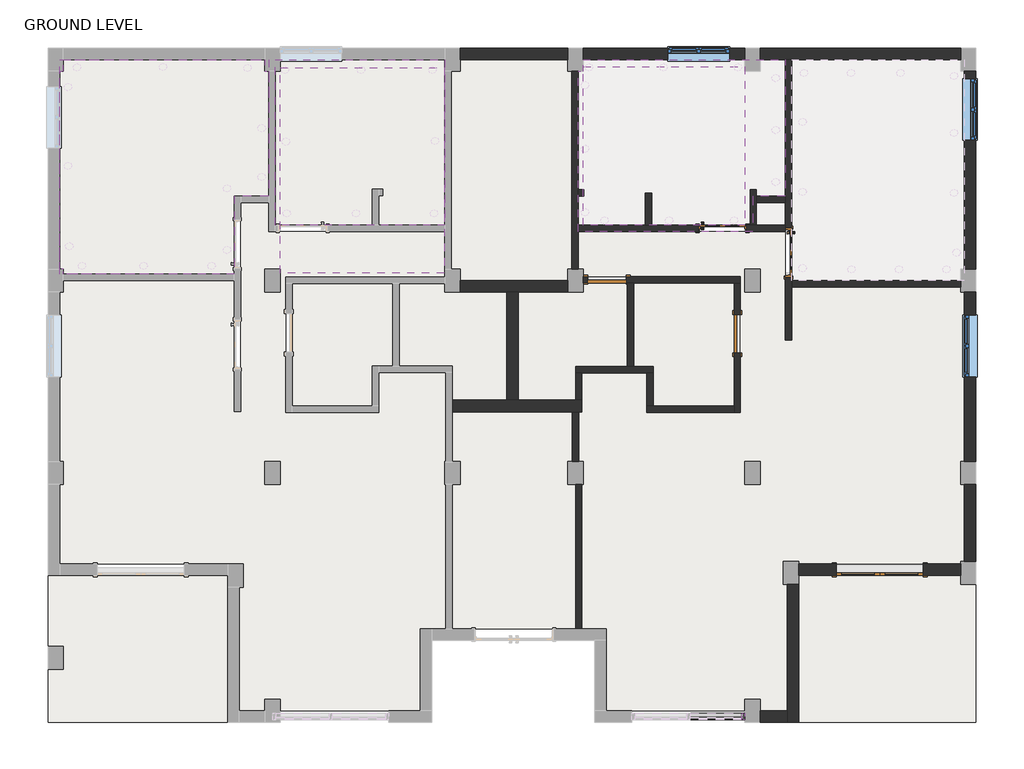
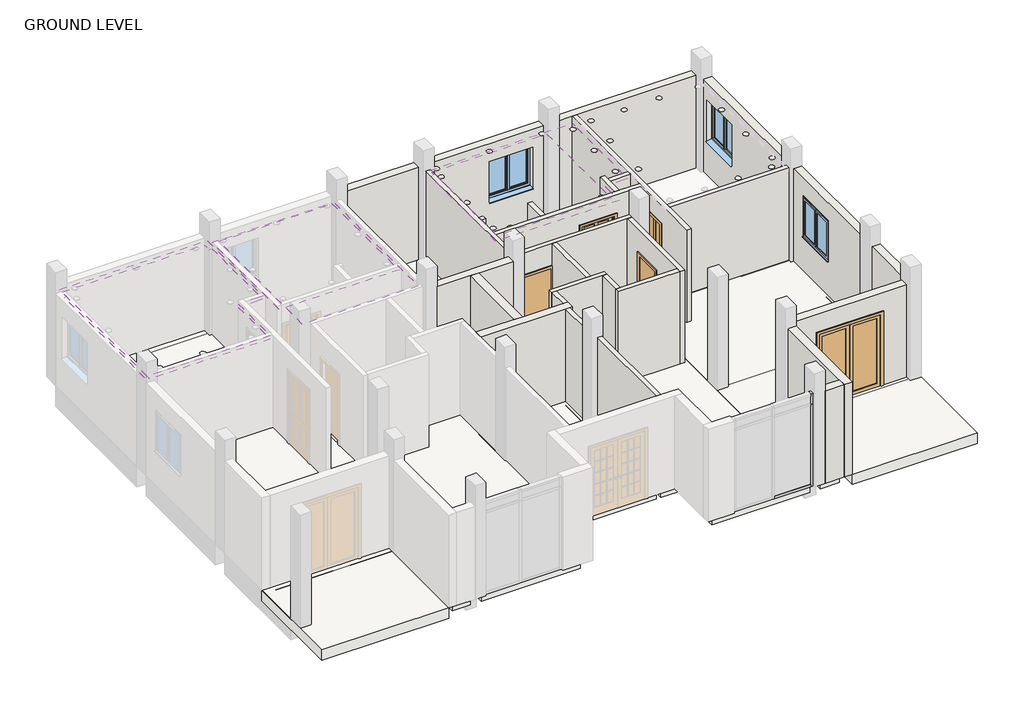
# One storey, part 2 of 5: 29 walls, 7 slabs, 6 coverings, 5 doors, 3 members, 3 windows.
"""IFC4 building model written with IfcOpenShell, lengths in millimetres."""

from ifc_helpers import new_model, si_unit, frame, origin, origin_with_axes, place, context, project, spatial, polyline, outline, extrude, faceted_brep, transform, mapped, element, save
from components import door_e52a3823, door_68a706ac, door_1fe7f57d, member_a1c24a98, member_ee409385, member_3c3dc66a, w2_0001_windows_4_x_4_9dec5fc7

model = new_model("IFC4")

# Units and contexts
model_context = context("Model", 3, world=origin())
ifc_project = project(units=[si_unit("LENGTHUNIT", "METRE", prefix="MILLI")], contexts=[model_context])

# Site, building, storey
site = spatial("IfcSite", under=ifc_project)
building = spatial("IfcBuilding", under=site)
storey = spatial("IfcBuildingStorey", under=building, Name="GROUND LEVEL", Elevation=0.0)

# Coverings
placement = place(None, origin())
element("IfcCovering", 1, ObjectType="white ceiling 6\"", at=placement, inside=storey, context=model_context, shape_type="SweptSolid", body=[
    extrude(outline(polyline([(-8916.1786397, -5702.2620333), (-8916.1786397, -1452.2061634), (-4776.7175798, -1452.2061634), (-4776.7175798, -4153.3104011), (-5462.5175798, -4153.3104011), (-5462.5175798, -5702.2620333), (-8916.1786397, -5702.2620333)])), frame((0.0, 0.0, 2641.6), z_axis=(0.0, 0.0, 1.0), x_axis=(1.0, 0.0, 0.0)), (0.0, 0.0, 1.0), 41.275),
])
element("IfcCovering", 2, ObjectType="white ceiling 6\"", at=placement, inside=storey, context=model_context, shape_type="SweptSolid", body=[
    extrude(outline(polyline([(-4852.9175798, -1452.2061634), (-4852.9175798, -1680.8061634), (-4776.7175798, -1680.8061634), (-4776.7175798, -4153.3104011), (-5462.5175798, -4153.3104011), (-5462.5175798, -5702.2620333), (-8839.9786397, -5702.2620333), (-8839.9786397, -5600.6620333), (-8916.1786397, -5600.6620333), (-8916.1786397, -1680.8061634), (-8839.9786397, -1680.8061634), (-8839.9786397, -1452.2061634), (-4852.9175798, -1452.2061634)]), holes=[polyline([(-8611.3786397, -5397.4620333), (-5767.3175798, -5397.4620333), (-5767.3175798, -3848.5104011), (-5081.5175798, -3848.5104011), (-5081.5175798, -1757.0061634), (-8611.3786397, -1757.0061634), (-8611.3786397, -5397.4620333)])]), frame((0.0, 0.0, 2540.0), z_axis=(0.0, 0.0, 1.0), x_axis=(1.0, 0.0, 0.0)), (0.0, 0.0, 1.0), 41.275),
])
element("IfcCovering", 3, ObjectType="white ceiling 6\"", at=placement, inside=storey, context=model_context, shape_type="SweptSolid", body=[
    extrude(outline(polyline([(-1296.9175798, -1452.2061634), (-1296.9175798, -4728.8061634), (-4649.7175798, -4728.8061634), (-4649.7175798, -1452.2061634), (-1296.9175798, -1452.2061634)]), holes=[polyline([(-1677.9175798, -1833.2061634), (-4268.7175798, -1833.2061634), (-4268.7175798, -4347.8061634), (-1677.9175798, -4347.8061634), (-1677.9175798, -1833.2061634)])]), frame((0.0, 0.0, 2540.0), z_axis=(0.0, 0.0, 1.0), x_axis=(1.0, 0.0, 0.0)), (0.0, 0.0, 1.0), 41.275),
])
element("IfcCovering", 4, ObjectType="white ceiling 6\"", at=placement, inside=storey, context=model_context, shape_type="SweptSolid", body=[
    extrude(outline(polyline([(5446.7824202, -1452.2061634), (5446.7824202, -1680.8061634), (5446.7824202, -4157.3061634), (4798.34348, -4157.3061634), (4798.34348, -4857.7120333), (1344.6824202, -4857.7120333), (1344.6824202, -1680.8061634), (1446.2824202, -1680.8061634), (1446.2824202, -1452.2061634), (5446.7824202, -1452.2061634)]), holes=[polyline([(1674.8824202, -4551.0061634), (4518.94348, -4551.0061634), (4518.94348, -3848.5104011), (5065.7824202, -3848.5104011), (5065.7824202, -1757.0061634), (1674.8824202, -1757.0061634), (1674.8824202, -4551.0061634)])]), frame((0.0, 0.0, 2540.0), z_axis=(0.0, 0.0, 1.0), x_axis=(1.0, 0.0, 0.0)), (0.0, 0.0, 1.0), 41.275),
])
element("IfcCovering", 5, ObjectType="white ceiling 6\"", at=placement, inside=storey, context=model_context, shape_type="SweptSolid", body=[
    extrude(outline(polyline([(1446.2303381, -4730.7120333), (1446.2303381, -1598.2561634), (4646.6303381, -1598.2561634), (4646.6303381, -4730.7120333), (1446.2303381, -4730.7120333)])), frame((0.0, 0.0, 2590.8), z_axis=(0.0, 0.0, 1.0), x_axis=(1.0, 0.0, 0.0)), (0.0, 0.0, 1.0), 41.275),
])
element("IfcCovering", 6, ObjectType="white ceiling 6\"", at=placement, inside=storey, context=model_context, shape_type="SweptSolid", body=[
    extrude(outline(polyline([(-4547.3786397, -5676.8620333), (-4547.3786397, -1617.3061634), (-1303.2675798, -1617.3061634), (-1303.2675798, -5676.8620333), (-4547.3786397, -5676.8620333)])), frame((0.0, 0.0, 2641.6), z_axis=(0.0, 0.0, 1.0), x_axis=(1.0, 0.0, 0.0)), (0.0, 0.0, 1.0), 41.275),
])

# Doors
door_shape = door_e52a3823(model_context)
element("IfcDoor", 7, ObjectType="Door-Double-Glass : 68\" x 84\"", at=placement, inside=storey, context=model_context, shape_type="MappedRepresentation", body=[
    mapped(door_shape, transform((7313.6824202, -11554.5807833, 0.0), x_axis=(-1.0, 0.0, 0.0), y_axis=(0.0, -1.0, 0.0), z_axis=(0.0, 0.0, 1.0))),
])
door_2_shape = door_68a706ac(model_context)
element("IfcDoor", 8, ObjectType="Door-Interior-Single-4_Panel-Wood : 36\" x 84\"", at=placement, inside=storey, context=model_context, shape_type="MappedRepresentation", body=[
    mapped(door_2_shape, transform((4202.1824202, -4789.1311634, 0.0), x_axis=(1.0, 0.0, 0.0), y_axis=(0.0, 1.0, 0.0), z_axis=(0.0, 0.0, 1.0))),
])
element("IfcDoor", 9, ObjectType="Door-Interior-Single-4_Panel-Wood : 36\" x 84\"", at=placement, inside=storey, context=model_context, shape_type="MappedRepresentation", body=[
    mapped(door_2_shape, transform((5513.4574202, -5274.9061634, 0.0), x_axis=(0.0, -1.0, 0.0), y_axis=(1.0, 0.0, 0.0), z_axis=(0.0, 0.0, 1.0))),
])
door_3_shape = door_1fe7f57d(model_context)
element("IfcDoor", 10, ObjectType="Single-Flush : 30\" x 80\"", at=placement, inside=storey, context=model_context, shape_type="MappedRepresentation", body=[
    mapped(door_3_shape, transform((1916.1824202, -5810.8691591, 0.0), x_axis=(-1.0, 0.0, 0.0), y_axis=(0.0, -1.0, 0.0), z_axis=(0.0, 0.0, 1.0))),
])
element("IfcDoor", 11, ObjectType="Single-Flush : 30\" x 80\"", at=placement, inside=storey, context=model_context, shape_type="MappedRepresentation", body=[
    mapped(door_3_shape, transform((4494.2824202, -6877.6691591, 0.0), x_axis=(0.0, 1.0, 0.0), y_axis=(-1.0, 0.0, 0.0), z_axis=(0.0, 0.0, 1.0))),
])

# Members
member_shape = member_a1c24a98(model_context)
element("IfcMember", 12, ObjectType="Rectangular Mullion : 2.5\" x 5\" rectangular", at=placement, inside=storey, context=model_context, shape_type="MappedRepresentation", body=[
    mapped(member_shape, transform((4583.1824202, -14462.5402089, 0.0), x_axis=(0.0, 0.0, -1.0), y_axis=(0.0, 1.0, 0.0), z_axis=(1.0, 0.0, 0.0))),
])
member_2_shape = member_ee409385(model_context)
element("IfcMember", 13, ObjectType="Rectangular Mullion : 2.5\" x 5\" rectangular", at=placement, inside=storey, context=model_context, shape_type="MappedRepresentation", body=[
    mapped(member_2_shape, transform((4646.6824202, -14462.5402089, 2438.4), x_axis=(1.0, 0.0, 0.0), y_axis=(0.0, 1.0, 0.0), z_axis=(0.0, 0.0, 1.0))),
])
member_3_shape = member_3c3dc66a(model_context)
element("IfcMember", 14, ObjectType="Rectangular Mullion : 2.5\" x 5\" rectangular", at=placement, inside=storey, context=model_context, shape_type="MappedRepresentation", body=[
    mapped(member_3_shape, transform((4646.6824202, -14462.5402089, 2743.2), x_axis=(1.0, 0.0, 0.0), y_axis=(0.0, 1.0, 0.0), z_axis=(0.0, 0.0, 1.0))),
])

# Slabs
element("IfcSlab", 15, ObjectType="TILE FLOORING 1'", at=placement, inside=storey, context=model_context, shape_type="SweptSolid", body=[
    extrude(outline(polyline([(-4315.5950401, -8312.1120333), (-4315.5950401, -5885.8942903), (-2325.6175798, -5885.8942903), (-2325.6175798, -7524.7120333), (-2728.0950401, -7524.7120333), (-2728.0950401, -8312.1120333), (-4315.5950401, -8312.1120333)])), frame((0.0, 0.0, -304.8), z_axis=(0.0, 0.0, 1.0), x_axis=(1.0, 0.0, 0.0)), (0.0, 0.0, 1.0), 304.8),
    extrude(outline(polyline([(-1296.9175798, -5885.8942903), (-1296.9175798, -6057.8620333), (-65.0175798, -6057.8620333), (-65.0175798, -8197.8120333), (-1144.5175798, -8197.8120333), (-1144.5175798, -7524.7120333), (-2198.6175798, -7524.7120333), (-2198.6175798, -5885.8942903), (-1296.9175798, -5885.8942903)])), frame((0.0, 0.0, -304.8), z_axis=(0.0, 0.0, 1.0), x_axis=(1.0, 0.0, 0.0)), (0.0, 0.0, 1.0), 304.8),
    extrude(outline(polyline([(1293.8824202, -8197.8120333), (163.5824202, -8197.8120333), (163.5824202, -6057.8620333), (1446.2824202, -6057.8620333), (1446.2824202, -5874.3691591), (2322.5824202, -5874.3691591), (2322.5824202, -7533.8890971), (1293.8824202, -7533.8890971), (1293.8824202, -8197.8120333)])), frame((0.0, 0.0, -304.8), z_axis=(0.0, 0.0, 1.0), x_axis=(1.0, 0.0, 0.0)), (0.0, 0.0, 1.0), 304.8),
    extrude(outline(polyline([(2449.5824202, -7533.8890971), (2449.5824202, -5874.3691591), (4430.7824202, -5874.3691591), (4430.7824202, -8312.7691591), (2830.5824202, -8312.7691591), (2830.5824202, -7533.8890971), (2449.5824202, -7533.8890971)])), frame((0.0, 0.0, -304.8), z_axis=(0.0, 0.0, 1.0), x_axis=(1.0, 0.0, 0.0)), (0.0, 0.0, 1.0), 304.8),
])
element("IfcSlab", 16, ObjectType="flooring 1'", at=placement, inside=storey, context=model_context, shape_type="SweptSolid", body=[
    extrude(outline(polyline([(-8916.1786397, -11442.6620333), (-8916.1786397, -9867.8620333), (-8839.9786397, -9867.8620333), (-8839.9786397, -9410.6620333), (-8916.1786397, -9410.6620333), (-8916.1786397, -6057.8620333), (-8839.9786397, -6057.8620333), (-8839.9786397, -5829.2620333), (-5462.5175798, -5829.2620333), (-5462.5175798, -8420.0620333), (-5335.5175798, -8420.0620333), (-5335.5175798, -4280.3104011), (-4776.7175798, -4280.3104011), (-4776.7175798, -4855.8061634), (-1296.9175798, -4855.8061634), (-1296.9175798, -5600.6620333), (-1296.9175798, -5758.8942903), (-4442.5950401, -5758.8942903), (-4442.5950401, -8439.1120333), (-2601.0950401, -8439.1120333), (-2601.0950401, -7651.7120333), (-1271.5175798, -7651.7120333), (-1271.5175798, -9410.6620333), (-1296.9175798, -9410.6620333), (-1296.9175798, -9867.8620333), (-1271.5175798, -9867.8620333), (-1271.5175798, -12722.6402089), (-1779.5175798, -12722.6402089), (-1779.5175798, -14348.2402089), (-4548.1175798, -14348.2402089), (-4548.1175798, -14119.6402089), (-4852.9175798, -14119.6402089), (-4852.9175798, -14348.2402089), (-5360.9175798, -14348.2402089), (-5360.9175798, -11899.8620333), (-5284.7175798, -11899.8620333), (-5284.7175798, -11442.6620333), (-5589.5175798, -11442.6620333), (-8916.1786397, -11442.6620333)])), frame((0.0, 0.0, -304.8), z_axis=(0.0, 0.0, 1.0), x_axis=(1.0, 0.0, 0.0)), (0.0, 0.0, 1.0), 304.8),
])
element("IfcSlab", 17, ObjectType="flooring 1'", at=placement, inside=storey, context=model_context, shape_type="SweptSolid", body=[
    extrude(outline(polyline([(5446.7824202, -4855.8061634), (5446.7824202, -6583.0061634), (5573.7824202, -6583.0061634), (5573.7824202, -5956.2620333), (8913.8824202, -5956.2620333), (8913.8824202, -6057.8620333), (8990.0824202, -6057.8620333), (8990.0824202, -9410.6620333), (8913.8824202, -9410.6620333), (8913.8824202, -9867.8620333), (8990.0824202, -9867.8620333), (8990.0824202, -11391.8620333), (8913.8824202, -11391.8620333), (8913.8824202, -11442.6620333), (5713.4824202, -11442.6620333), (5713.4824202, -11391.8620333), (5408.6824202, -11391.8620333), (5408.6824202, -11849.0620333), (5484.8824202, -11849.0620333), (5484.8824202, -14348.2402089), (4951.4824202, -14348.2402089), (4951.4824202, -14119.6402089), (4646.6824202, -14119.6402089), (4646.6824202, -14348.2402089), (1903.4824202, -14348.2402089), (1903.4824202, -12722.6402089), (1420.8824202, -12722.6402089), (1420.8824202, -9867.8620333), (1446.2824202, -9867.8620333), (1446.2824202, -9410.6620333), (1357.3824202, -9410.6620333), (1357.3824202, -8426.4120333), (1420.8824202, -8426.4120333), (1420.8824202, -7660.8890971), (2703.5824202, -7660.8890971), (2703.5824202, -8439.7691591), (4557.7824202, -8439.7691591), (4557.7824202, -5747.3691591), (1446.2824202, -5747.3691591), (1446.2824202, -5600.6620333), (1344.6824202, -5600.6620333), (1344.6824202, -4855.8061634), (5446.7824202, -4855.8061634)])), frame((0.0, 0.0, -304.8), z_axis=(0.0, 0.0, 1.0), x_axis=(1.0, 0.0, 0.0)), (0.0, 0.0, 1.0), 304.8),
])
element("IfcSlab", 18, ObjectType="flooring 1'", at=placement, inside=storey, context=model_context, shape_type="SweptSolid", body=[
    extrude(outline(polyline([(-8839.9786397, -1680.8061634), (-8839.9786397, -1452.2061634), (-4852.9175798, -1452.2061634), (-4852.9175798, -1680.8061634), (-4776.7175798, -1680.8061634), (-4776.7175798, -4153.3104011), (-5462.5175798, -4153.3104011), (-5462.5175798, -5702.2620333), (-8839.9786397, -5702.2620333), (-8839.9786397, -5600.6620333), (-8916.1786397, -5600.6620333), (-8916.1786397, -1680.8061634), (-8839.9786397, -1680.8061634)])), frame((0.0, 0.0, -304.8), z_axis=(0.0, 0.0, 1.0), x_axis=(1.0, 0.0, 0.0)), (0.0, 0.0, 1.0), 304.8),
    extrude(outline(polyline([(-2732.0175798, -4728.8061634), (-4649.7175798, -4728.8061634), (-4649.7175798, -1680.8061634), (-4548.1175798, -1680.8061634), (-4548.1175798, -1452.2061634), (-1296.9175798, -1452.2061634), (-1296.9175798, -4728.8061634), (-2605.0175798, -4728.8061634), (-2605.0175798, -4144.6061634), (-2516.1175798, -4144.6061634), (-2516.1175798, -4017.6061634), (-2732.0175798, -4017.6061634), (-2732.0175798, -4728.8061634)])), frame((0.0, 0.0, -304.8), z_axis=(0.0, 0.0, 1.0), x_axis=(1.0, 0.0, 0.0)), (0.0, 0.0, 1.0), 304.8),
])
element("IfcSlab", 19, ObjectType="flooring 1'", at=placement, inside=storey, context=model_context, shape_type="SweptSolid", body=[
    extrude(outline(polyline([(1141.4824202, -1452.2061634), (1141.4824202, -1680.8061634), (1217.6824202, -1680.8061634), (1217.6824202, -5600.6620333), (1141.4824202, -5600.6620333), (1141.4824202, -5829.2620333), (-992.1175798, -5829.2620333), (-992.1175798, -5600.6620333), (-1169.9175798, -5600.6620333), (-1169.9175798, -1680.8061634), (-992.1175798, -1680.8061634), (-992.1175798, -1452.2061634), (1141.4824202, -1452.2061634)])), frame((0.0, 0.0, -304.8), z_axis=(0.0, 0.0, 1.0), x_axis=(1.0, 0.0, 0.0)), (0.0, 0.0, 1.0), 304.8),
])
element("IfcSlab", 20, ObjectType="flooring 1'", at=placement, inside=storey, context=model_context, shape_type="SweptSolid", body=[
    extrude(outline(polyline([(1293.8824202, -12722.6402089), (-1144.5175798, -12722.6402089), (-1144.5175798, -9867.8620333), (-992.1175798, -9867.8620333), (-992.1175798, -9410.6620333), (-1144.5175798, -9410.6620333), (-1144.5175798, -8426.4120333), (1230.3824202, -8426.4120333), (1230.3824202, -9410.6620333), (1141.4824202, -9410.6620333), (1141.4824202, -9867.8620333), (1293.8824202, -9867.8620333), (1293.8824202, -12722.6402089)])), frame((0.0, 0.0, -304.8), z_axis=(0.0, 0.0, 1.0), x_axis=(1.0, 0.0, 0.0)), (0.0, 0.0, 1.0), 304.8),
])
element("IfcSlab", 21, ObjectType="flooring 1'", at=placement, inside=storey, context=model_context, shape_type="SweptSolid", body=[
    extrude(outline(polyline([(-5589.5175798, -11671.2620333), (-5589.5175798, -14576.8402089), (-9144.7786397, -14576.8402089), (-9144.7786397, -11671.2620333), (-5589.5175798, -11671.2620333)])), frame((0.0, 0.0, -304.8), z_axis=(0.0, 0.0, 1.0), x_axis=(1.0, 0.0, 0.0)), (0.0, 0.0, 1.0), 304.8),
    extrude(outline(polyline([(9218.6824202, -11671.2620333), (9218.6824202, -14576.8402089), (5713.4824202, -14576.8402089), (5713.4824202, -11671.2620333), (9218.6824202, -11671.2620333)])), frame((0.0, 0.0, -304.8), z_axis=(0.0, 0.0, 1.0), x_axis=(1.0, 0.0, 0.0)), (0.0, 0.0, 1.0), 304.8),
])

# Walls
element("IfcWall", 22, ObjectType="EXTERIOR WALL 9\"", at=placement, inside=storey, context=model_context, shape_type="SweptSolid", body=[
    extrude(outline(polyline([(1141.4824202, -1452.2061634), (-992.1175798, -1452.2061634), (-992.1175798, -1223.6061634), (1141.4824202, -1223.6061634), (1141.4824202, -1452.2061634)])), origin_with_axes(), (0.0, 0.0, 1.0), 2743.2),
])
element("IfcWall", 23, ObjectType="EXTERIOR WALL 9\"", at=placement, inside=storey, context=model_context, shape_type="SweptSolid", body=[
    extrude(outline(polyline([(0.0, 1446.2824202), (0.0, 4646.6824202), (2743.2, 4646.6824202), (2743.2, 1446.2824202), (0.0, 1446.2824202)]), holes=[polyline([(1000.0, 4341.8824202), (1000.0, 3122.6824202), (2219.2, 3122.6824202), (2219.2, 4341.8824202), (1000.0, 4341.8824202)])]), frame((0.0, -1452.2061634, 0.0), z_axis=(0.0, 1.0, 0.0), x_axis=(0.0, 0.0, 1.0)), (0.0, 0.0, 1.0), 228.6),
])
element("IfcWall", 24, ObjectType="EXTERIOR WALL 9\"", at=placement, inside=storey, context=model_context, shape_type="Brep", body=[
    faceted_brep([(4951.4824202, -1452.2061634, 0.0), (5446.7824202, -1452.2061634, 0.0), (5573.7824202, -1452.2061634, 0.0), (8913.8824202, -1452.2061634, 0.0), (8913.8824202, -1452.2061634, 2743.2), (5573.7824202, -1452.2061634, 2743.2), (5446.7824202, -1452.2061634, 2743.2), (4951.4824202, -1452.2061634, 2743.2), (4951.4824202, -1223.6061634, 0.0), (4951.4824202, -1223.6061634, 2743.2), (8913.8824202, -1223.6061634, 2743.2), (8913.8824202, -1223.6061634, 0.0)], [[[0, 1, 2, 3, 4, 5, 6, 7]], [[8, 9, 10, 11]], [[3, 2, 1, 0, 8, 11]], [[4, 3, 11, 10]], [[7, 6, 5, 4, 10, 9]], [[0, 7, 9, 8]]]),
])
element("IfcWall", 25, ObjectType="EXTERIOR WALL 9\"", at=placement, inside=storey, context=model_context, shape_type="SweptSolid", body=[
    extrude(outline(polyline([(-1680.8061634, 0.0), (-5600.6620333, 0.0), (-5600.6620333, 2743.2), (-1680.8061634, 2743.2), (-1680.8061634, 0.0)]), holes=[polyline([(-3052.4061634, 1000.0), (-1833.2061634, 1000.0), (-1833.2061634, 2219.2), (-3052.4061634, 2219.2), (-3052.4061634, 1000.0)])]), frame((8990.0824202, 0.0, 0.0), z_axis=(1.0, 0.0, 0.0), x_axis=(0.0, 1.0, 0.0)), (0.0, 0.0, 1.0), 228.6),
])
element("IfcWall", 26, ObjectType="EXTERIOR WALL 9\"", at=placement, inside=storey, context=model_context, shape_type="SweptSolid", body=[
    extrude(outline(polyline([(-6057.8620333, 0.0), (-9410.6620333, 0.0), (-9410.6620333, 2743.2), (-6057.8620333, 2743.2), (-6057.8620333, 0.0)]), holes=[polyline([(-6515.0620333, 1000.0), (-6515.0620333, 2219.2), (-7734.2620333, 2219.2), (-7734.2620333, 1000.0), (-6515.0620333, 1000.0)])]), frame((8990.0824202, 0.0, 0.0), z_axis=(1.0, 0.0, 0.0), x_axis=(0.0, 1.0, 0.0)), (0.0, 0.0, 1.0), 228.6),
])
element("IfcWall", 27, ObjectType="EXTERIOR WALL 9\"", at=placement, inside=storey, context=model_context, shape_type="SweptSolid", body=[
    extrude(outline(polyline([(8990.0824202, -11391.8620333), (8990.0824202, -9867.8620333), (9218.6824202, -9867.8620333), (9218.6824202, -11391.8620333), (8990.0824202, -11391.8620333)])), origin_with_axes(), (0.0, 0.0, 1.0), 2743.2),
])
element("IfcWall", 28, ObjectType="EXTERIOR WALL 9\"", at=placement, inside=storey, context=model_context, shape_type="SweptSolid", body=[
    extrude(outline(polyline([(2743.2, 5713.4824202), (0.0, 5713.4824202), (0.0, 6450.0824202), (2133.6, 6450.0824202), (2133.6, 8177.2824202), (0.0, 8177.2824202), (0.0, 8913.8824202), (2743.2, 8913.8824202), (2743.2, 5713.4824202)])), frame((0.0, -11671.2620333, 0.0), z_axis=(0.0, 1.0, 0.0), x_axis=(0.0, 0.0, 1.0)), (0.0, 0.0, 1.0), 228.6),
])
element("IfcWall", 29, ObjectType="EXTERIOR WALL 9\"", at=placement, inside=storey, context=model_context, shape_type="Brep", body=[
    faceted_brep([(5484.8824202, -11849.0620333, 0.0), (5484.8824202, -14348.2402089, 0.0), (5484.8824202, -14576.8402089, 0.0), (5484.8824202, -14576.8402089, 2743.2), (5484.8824202, -14348.2402089, 2743.2), (5484.8824202, -11849.0620333, 2743.2), (5713.4824202, -11849.0620333, 0.0), (5713.4824202, -11849.0620333, 2743.2), (5713.4824202, -14576.8402089, 2743.2), (5713.4824202, -14576.8402089, 0.0)], [[[0, 1, 2, 3, 4, 5]], [[6, 7, 8, 9]], [[2, 1, 0, 6, 9]], [[5, 4, 3, 8, 7]], [[0, 5, 7, 6]], [[3, 2, 9, 8]]]),
])
element("IfcWall", 30, ObjectType="EXTERIOR WALL 9\"", at=placement, inside=storey, context=model_context, shape_type="SweptSolid", body=[
    extrude(outline(polyline([(5484.8824202, -14576.8402089), (4951.4824202, -14576.8402089), (4951.4824202, -14348.2402089), (5484.8824202, -14348.2402089), (5484.8824202, -14576.8402089)])), origin_with_axes(), (0.0, 0.0, 1.0), 2743.2),
])
element("IfcWall", 31, ObjectType="EXTERIOR WALL 9\"", at=placement, inside=storey, context=model_context, shape_type="Brep", body=[
    faceted_brep([(1141.4824202, -5829.2620333, 0.0), (-992.1175798, -5829.2620333, 0.0), (-992.1175798, -5829.2620333, 2743.2), (1141.4824202, -5829.2620333, 2743.2), (1141.4824202, -6057.8620333, 0.0), (1141.4824202, -6057.8620333, 2743.2), (163.5824202, -6057.8620333, 2743.2), (-65.0175798, -6057.8620333, 2743.2), (-992.1175798, -6057.8620333, 2743.2), (-992.1175798, -6057.8620333, 0.0), (-65.0175798, -6057.8620333, 0.0), (163.5824202, -6057.8620333, 0.0)], [[[0, 1, 2, 3]], [[4, 5, 6, 7, 8, 9, 10, 11]], [[1, 0, 4, 11, 10, 9]], [[2, 1, 9, 8]], [[3, 2, 8, 7, 6, 5]], [[0, 3, 5, 4]]]),
])
element("IfcWall", 32, ObjectType="EXTERIOR WALL 9\"", at=placement, inside=storey, context=model_context, shape_type="SweptSolid", body=[
    extrude(outline(polyline([(-65.0175798, -8197.8120333), (-65.0175798, -6057.8620333), (163.5824202, -6057.8620333), (163.5824202, -8197.8120333), (-65.0175798, -8197.8120333)])), origin_with_axes(), (0.0, 0.0, 1.0), 2743.2),
])
element("IfcWall", 33, ObjectType="EXTERIOR WALL 9\"", at=placement, inside=storey, context=model_context, shape_type="Brep", body=[
    faceted_brep([(-1144.5175798, -8426.4120333, 0.0), (1230.3824202, -8426.4120333, 0.0), (1357.3824202, -8426.4120333, 0.0), (1420.8824202, -8426.4120333, 0.0), (1420.8824202, -8426.4120333, 2743.2), (1357.3824202, -8426.4120333, 2743.2), (1230.3824202, -8426.4120333, 2743.2), (-1144.5175798, -8426.4120333, 2743.2), (-1144.5175798, -8197.8120333, 0.0), (-1144.5175798, -8197.8120333, 2743.2), (-65.0175798, -8197.8120333, 2743.2), (163.5824202, -8197.8120333, 2743.2), (1293.8824202, -8197.8120333, 2743.2), (1420.8824202, -8197.8120333, 2743.2), (1420.8824202, -8197.8120333, 0.0), (1293.8824202, -8197.8120333, 0.0), (163.5824202, -8197.8120333, 0.0), (-65.0175798, -8197.8120333, 0.0)], [[[0, 1, 2, 3, 4, 5, 6, 7]], [[8, 9, 10, 11, 12, 13, 14, 15, 16, 17]], [[3, 2, 1, 0, 8, 17, 16, 15, 14]], [[7, 6, 5, 4, 13, 12, 11, 10, 9]], [[0, 7, 9, 8]], [[4, 3, 14, 13]]]),
])
element("IfcWall", 34, ObjectType="INTERIOR WALL 5\"", at=placement, inside=storey, context=model_context, shape_type="Brep", body=[
    faceted_brep([(1217.6824202, -1680.8061634, 0.0), (1217.6824202, -5600.6620333, 0.0), (1217.6824202, -5600.6620333, 2743.2), (1217.6824202, -1680.8061634, 2743.2), (1344.6824202, -1680.8061634, 0.0), (1344.6824202, -1680.8061634, 2743.2), (1344.6824202, -4030.3061634, 2743.2), (1344.6824202, -4157.3061634, 2743.2), (1344.6824202, -4728.8061634, 2743.2), (1344.6824202, -4855.8061634, 2743.2), (1344.6824202, -5600.6620333, 2743.2), (1344.6824202, -5600.6620333, 0.0), (1344.6824202, -4855.8061634, 0.0), (1344.6824202, -4728.8061634, 0.0), (1344.6824202, -4157.3061634, 0.0), (1344.6824202, -4030.3061634, 0.0)], [[[0, 1, 2, 3]], [[4, 5, 6, 7, 8, 9, 10, 11, 12, 13, 14, 15]], [[1, 0, 4, 15, 14, 13, 12, 11]], [[2, 1, 11, 10]], [[3, 2, 10, 9, 8, 7, 6, 5]], [[0, 3, 5, 4]]]),
])
element("IfcWall", 35, ObjectType="INTERIOR WALL 5\"", at=placement, inside=storey, context=model_context, shape_type="Brep", body=[
    faceted_brep([(5446.7824202, -4855.8061634, 2743.2), (1344.6824202, -4855.8061634, 2743.2), (1344.6824202, -4855.8061634, 0.0), (3719.5824202, -4855.8061634, 0.0), (3719.5824202, -4855.8061634, 2159.0), (4684.7824202, -4855.8061634, 2159.0), (4684.7824202, -4855.8061634, 0.0), (5446.7824202, -4855.8061634, 0.0), (1344.6824202, -4728.8061634, 2743.2), (2678.1824202, -4728.8061634, 2743.2), (2805.1824202, -4728.8061634, 2743.2), (4748.2824202, -4728.8061634, 2743.2), (4875.2824202, -4728.8061634, 2743.2), (5446.7824202, -4728.8061634, 2743.2), (5446.7824202, -4728.8061634, 0.0), (4875.2824202, -4728.8061634, 0.0), (4748.2824202, -4728.8061634, 0.0), (4684.7824202, -4728.8061634, 0.0), (4684.7824202, -4728.8061634, 2159.0), (3719.5824202, -4728.8061634, 2159.0), (3719.5824202, -4728.8061634, 0.0), (2805.1824202, -4728.8061634, 0.0), (2678.1824202, -4728.8061634, 0.0), (1344.6824202, -4728.8061634, 0.0)], [[[0, 1, 2, 3, 4, 5, 6, 7]], [[8, 9, 10, 11, 12, 13, 14, 15, 16, 17, 18, 19, 20, 21, 22, 23]], [[2, 23, 22, 21, 20, 3]], [[14, 7, 6, 17, 16, 15]], [[1, 0, 13, 12, 11, 10, 9, 8]], [[2, 1, 8, 23]], [[0, 7, 14, 13]], [[5, 18, 17, 6]], [[18, 5, 4, 19]], [[19, 4, 3, 20]]]),
])
element("IfcWall", 36, ObjectType="INTERIOR WALL 5\"", at=placement, inside=storey, context=model_context, shape_type="Brep", body=[
    faceted_brep([(4875.2824202, -4728.8061634, 0.0), (4875.2824202, -4284.3061634, 0.0), (4875.2824202, -4157.3061634, 0.0), (4875.2824202, -4030.3061634, 0.0), (4875.2824202, -4030.3061634, 2743.2), (4875.2824202, -4157.3061634, 2743.2), (4875.2824202, -4284.3061634, 2743.2), (4875.2824202, -4728.8061634, 2743.2), (4748.2824202, -4728.8061634, 0.0), (4748.2824202, -4728.8061634, 2743.2), (4748.2824202, -4030.3061634, 2743.2), (4748.2824202, -4030.3061634, 0.0)], [[[0, 1, 2, 3, 4, 5, 6, 7]], [[8, 9, 10, 11]], [[3, 2, 1, 0, 8, 11]], [[4, 3, 11, 10]], [[7, 6, 5, 4, 10, 9]], [[0, 7, 9, 8]]]),
])
element("IfcWall", 37, ObjectType="INTERIOR WALL 5\"", at=placement, inside=storey, context=model_context, shape_type="SweptSolid", body=[
    extrude(outline(polyline([(5446.7824202, -4284.3061634), (4875.2824202, -4284.3061634), (4875.2824202, -4157.3061634), (5446.7824202, -4157.3061634), (5446.7824202, -4284.3061634)])), origin_with_axes(), (0.0, 0.0, 1.0), 2743.2),
])
element("IfcWall", 38, ObjectType="INTERIOR WALL 5\"", at=placement, inside=storey, context=model_context, shape_type="Brep", body=[
    faceted_brep([(5446.7824202, -7002.1061634, 0.0), (5446.7824202, -7002.1061634, 2743.2), (5446.7824202, -4855.8061634, 2743.2), (5446.7824202, -4728.8061634, 2743.2), (5446.7824202, -4284.3061634, 2743.2), (5446.7824202, -4157.3061634, 2743.2), (5446.7824202, -1452.2061634, 2743.2), (5446.7824202, -1452.2061634, 0.0), (5446.7824202, -4157.3061634, 0.0), (5446.7824202, -4284.3061634, 0.0), (5446.7824202, -4728.8061634, 0.0), (5446.7824202, -4792.3061634, 0.0), (5446.7824202, -4792.3061634, 2159.0), (5446.7824202, -5757.5061634, 2159.0), (5446.7824202, -5757.5061634, 0.0), (5573.7824202, -7002.1061634, 2743.2), (5573.7824202, -7002.1061634, 0.0), (5573.7824202, -5956.2620333, 0.0), (5573.7824202, -5829.2620333, 0.0), (5573.7824202, -5757.5061634, 0.0), (5573.7824202, -5757.5061634, 2159.0), (5573.7824202, -4792.3061634, 2159.0), (5573.7824202, -4792.3061634, 0.0), (5573.7824202, -1452.2061634, 0.0), (5573.7824202, -1452.2061634, 2743.2), (5573.7824202, -5829.2620333, 2743.2), (5573.7824202, -5956.2620333, 2743.2)], [[[0, 1, 2, 3, 4, 5, 6, 7, 8, 9, 10, 11, 12, 13, 14]], [[15, 16, 17, 18, 19, 20, 21, 22, 23, 24, 25, 26]], [[16, 0, 14, 19, 18, 17]], [[7, 23, 22, 11, 10, 9, 8]], [[1, 0, 16, 15]], [[6, 5, 4, 3, 2, 1, 15, 26, 25, 24]], [[7, 6, 24, 23]], [[13, 20, 19, 14]], [[20, 13, 12, 21]], [[21, 12, 11, 22]]]),
])
element("IfcWall", 39, ObjectType="INTERIOR WALL 5\"", at=placement, inside=storey, context=model_context, shape_type="SweptSolid", body=[
    extrude(outline(polyline([(5573.7824202, -5829.2620333), (8913.8824202, -5829.2620333), (8913.8824202, -5956.2620333), (5573.7824202, -5956.2620333), (5573.7824202, -5829.2620333)])), origin_with_axes(), (0.0, 0.0, 1.0), 2743.2),
])
element("IfcWall", 40, ObjectType="INTERIOR WALL 5\"", at=placement, inside=storey, context=model_context, shape_type="SweptSolid", body=[
    extrude(outline(polyline([(2805.1824202, -4093.8061634), (2805.1824202, -4728.8061634), (2678.1824202, -4728.8061634), (2678.1824202, -4093.8061634), (2805.1824202, -4093.8061634)])), origin_with_axes(), (0.0, 0.0, 1.0), 2743.2),
])
element("IfcWall", 41, ObjectType="INTERIOR WALL 5\"", at=placement, inside=storey, context=model_context, shape_type="SweptSolid", body=[
    extrude(outline(polyline([(1458.9824202, -4157.3061634), (1344.6824202, -4157.3061634), (1344.6824202, -4030.3061634), (1458.9824202, -4030.3061634), (1458.9824202, -4157.3061634)])), origin_with_axes(), (0.0, 0.0, 1.0), 2743.2),
])
element("IfcWall", 42, ObjectType="INTERIOR WALL 5\"", at=placement, inside=storey, context=model_context, shape_type="Brep", body=[
    faceted_brep([(1535.1824202, -5747.3691591, 2032.0), (1535.1824202, -5747.3691591, 0.0), (1446.2824202, -5747.3691591, 0.0), (1446.2824202, -5747.3691591, 2743.2), (4557.7824202, -5747.3691591, 2743.2), (4557.7824202, -5747.3691591, 0.0), (2297.1824202, -5747.3691591, 0.0), (2297.1824202, -5747.3691591, 2032.0), (1446.2824202, -5874.3691591, 0.0), (1535.1824202, -5874.3691591, 0.0), (1535.1824202, -5874.3691591, 2032.0), (2297.1824202, -5874.3691591, 2032.0), (2297.1824202, -5874.3691591, 0.0), (2322.5824202, -5874.3691591, 0.0), (2449.5824202, -5874.3691591, 0.0), (4430.7824202, -5874.3691591, 0.0), (4557.7824202, -5874.3691591, 0.0), (4557.7824202, -5874.3691591, 2743.2), (4430.7824202, -5874.3691591, 2743.2), (2449.5824202, -5874.3691591, 2743.2), (2322.5824202, -5874.3691591, 2743.2), (1446.2824202, -5874.3691591, 2743.2)], [[[0, 1, 2, 3, 4, 5, 6, 7]], [[8, 9, 10, 11, 12, 13, 14, 15, 16, 17, 18, 19, 20, 21]], [[6, 5, 16, 15, 14, 13, 12]], [[2, 1, 9, 8]], [[3, 2, 8, 21]], [[4, 3, 21, 20, 19, 18, 17]], [[5, 4, 17, 16]], [[10, 9, 1, 0]], [[11, 10, 0, 7]], [[12, 11, 7, 6]]]),
])
element("IfcWall", 43, ObjectType="INTERIOR WALL 5\"", at=placement, inside=storey, context=model_context, shape_type="Brep", body=[
    faceted_brep([(4430.7824202, -5874.3691591, 0.0), (4430.7824202, -6496.6691591, 0.0), (4430.7824202, -6496.6691591, 2032.0), (4430.7824202, -7258.6691591, 2032.0), (4430.7824202, -7258.6691591, 0.0), (4430.7824202, -8312.7691591, 0.0), (4430.7824202, -8439.7691591, 0.0), (4430.7824202, -8439.7691591, 2743.2), (4430.7824202, -8312.7691591, 2743.2), (4430.7824202, -5874.3691591, 2743.2), (4557.7824202, -6496.6691591, 2032.0), (4557.7824202, -6496.6691591, 0.0), (4557.7824202, -5874.3691591, 0.0), (4557.7824202, -5874.3691591, 2743.2), (4557.7824202, -8439.7691591, 2743.2), (4557.7824202, -8439.7691591, 0.0), (4557.7824202, -7258.6691591, 0.0), (4557.7824202, -7258.6691591, 2032.0)], [[[0, 1, 2, 3, 4, 5, 6, 7, 8, 9]], [[10, 11, 12, 13, 14, 15, 16, 17]], [[16, 15, 6, 5, 4]], [[12, 11, 1, 0]], [[9, 8, 7, 14, 13]], [[0, 9, 13, 12]], [[7, 6, 15, 14]], [[2, 1, 11, 10]], [[3, 2, 10, 17]], [[4, 3, 17, 16]]]),
])
element("IfcWall", 44, ObjectType="INTERIOR WALL 5\"", at=placement, inside=storey, context=model_context, shape_type="Brep", body=[
    faceted_brep([(4430.7824202, -8312.7691591, 0.0), (2830.5824202, -8312.7691591, 0.0), (2703.5824202, -8312.7691591, 0.0), (2703.5824202, -8312.7691591, 2743.2), (2830.5824202, -8312.7691591, 2743.2), (4430.7824202, -8312.7691591, 2743.2), (4430.7824202, -8439.7691591, 0.0), (4430.7824202, -8439.7691591, 2743.2), (2703.5824202, -8439.7691591, 2743.2), (2703.5824202, -8439.7691591, 0.0)], [[[0, 1, 2, 3, 4, 5]], [[6, 7, 8, 9]], [[2, 1, 0, 6, 9]], [[5, 4, 3, 8, 7]], [[0, 5, 7, 6]], [[3, 2, 9, 8]]]),
])
element("IfcWall", 45, ObjectType="INTERIOR WALL 5\"", at=placement, inside=storey, context=model_context, shape_type="SweptSolid", body=[
    extrude(outline(polyline([(2830.5824202, -7660.8890971), (2830.5824202, -8312.7691591), (2703.5824202, -8312.7691591), (2703.5824202, -7660.8890971), (2830.5824202, -7660.8890971)])), origin_with_axes(), (0.0, 0.0, 1.0), 2743.2),
])
element("IfcWall", 46, ObjectType="INTERIOR WALL 5\"", at=placement, inside=storey, context=model_context, shape_type="Brep", body=[
    faceted_brep([(2830.5824202, -7533.8890971, 0.0), (2449.5824202, -7533.8890971, 0.0), (2322.5824202, -7533.8890971, 0.0), (1293.8824202, -7533.8890971, 0.0), (1293.8824202, -7533.8890971, 2743.2), (2322.5824202, -7533.8890971, 2743.2), (2449.5824202, -7533.8890971, 2743.2), (2830.5824202, -7533.8890971, 2743.2), (2830.5824202, -7660.8890971, 0.0), (2830.5824202, -7660.8890971, 2743.2), (2703.5824202, -7660.8890971, 2743.2), (1420.8824202, -7660.8890971, 2743.2), (1293.8824202, -7660.8890971, 2743.2), (1293.8824202, -7660.8890971, 0.0), (1420.8824202, -7660.8890971, 0.0), (2703.5824202, -7660.8890971, 0.0)], [[[0, 1, 2, 3, 4, 5, 6, 7]], [[8, 9, 10, 11, 12, 13, 14, 15]], [[3, 2, 1, 0, 8, 15, 14, 13]], [[7, 6, 5, 4, 12, 11, 10, 9]], [[0, 7, 9, 8]], [[4, 3, 13, 12]]]),
])
element("IfcWall", 47, ObjectType="INTERIOR WALL 5\"", at=placement, inside=storey, context=model_context, shape_type="SweptSolid", body=[
    extrude(outline(polyline([(1293.8824202, -8197.8120333), (1293.8824202, -7660.8890971), (1420.8824202, -7660.8890971), (1420.8824202, -8197.8120333), (1293.8824202, -8197.8120333)])), origin_with_axes(), (0.0, 0.0, 1.0), 2743.2),
])
element("IfcWall", 48, ObjectType="INTERIOR WALL 5\"", at=placement, inside=storey, context=model_context, shape_type="SweptSolid", body=[
    extrude(outline(polyline([(2322.5824202, -7533.8890971), (2322.5824202, -5874.3691591), (2449.5824202, -5874.3691591), (2449.5824202, -7533.8890971), (2322.5824202, -7533.8890971)])), origin_with_axes(), (0.0, 0.0, 1.0), 2743.2),
])
element("IfcWall", 49, ObjectType="INTERIOR WALL 5\"", at=placement, inside=storey, context=model_context, shape_type="SweptSolid", body=[
    extrude(outline(polyline([(1293.8824202, -12722.6402089), (1293.8824202, -9867.8620333), (1420.8824202, -9867.8620333), (1420.8824202, -12722.6402089), (1293.8824202, -12722.6402089)])), origin_with_axes(), (0.0, 0.0, 1.0), 2743.2),
])
element("IfcWall", 50, ObjectType="INTERIOR WALL 5\"", at=placement, inside=storey, context=model_context, shape_type="SweptSolid", body=[
    extrude(outline(polyline([(1357.3824202, -8426.4120333), (1357.3824202, -9410.6620333), (1230.3824202, -9410.6620333), (1230.3824202, -8426.4120333), (1357.3824202, -8426.4120333)])), origin_with_axes(), (0.0, 0.0, 1.0), 2743.2),
])

# Windows
w2_0001_windows_4_x_4_shape = w2_0001_windows_4_x_4_9dec5fc7(model_context)
element("IfcWindow", 51, ObjectType="w2.0001 : WINDOWS 4' X 4'", at=placement, inside=storey, context=model_context, shape_type="MappedRepresentation", body=[
    mapped(w2_0001_windows_4_x_4_shape, transform((9104.3824202, -7124.6620333, 0.0), x_axis=(0.0, -1.0, 0.0), y_axis=(1.0, 0.0, 0.0), z_axis=(0.0, 0.0, 1.0))),
])
element("IfcWindow", 52, ObjectType="w2.0001 : WINDOWS 4' X 4'", at=placement, inside=storey, context=model_context, shape_type="MappedRepresentation", body=[
    mapped(w2_0001_windows_4_x_4_shape, transform((9104.3824202, -2442.8061634, 0.0), x_axis=(0.0, 1.0, 0.0), y_axis=(-1.0, 0.0, 0.0), z_axis=(0.0, 0.0, 1.0))),
])
element("IfcWindow", 53, ObjectType="w2.0001 : WINDOWS 4' X 4'", at=placement, inside=storey, context=model_context, shape_type="MappedRepresentation", body=[
    mapped(w2_0001_windows_4_x_4_shape, transform((3732.2824202, -1337.9061634, 0.0), x_axis=(-1.0, 0.0, 0.0), y_axis=(0.0, -1.0, 0.0), z_axis=(0.0, 0.0, 1.0))),
])

save(model, "model.ifc")

# Revit data of these elements
# Type "white ceiling 6\""
#   Assembly Code = "C3030220"
#   built-in parameter 1002203 = 1 (stored number, unit not read)
#   built-in parameter 1002202 = 1 (stored number, unit not read)
#   Layers, outside or top first: 0' - 1" "white ceiling" (function 1); 0' - 0 5/8" "white ceiling" (function 5)
# Type "Door-Double-Glass : 68\" x 84\""
#   Type Mark = "11"
#   Construction Type Id = "opn-d45"
#   Assembly Code = "C1020"
#   Analytic Construction = "Wood frame, double glass door "
#   W = 2' - 10"
#   Thickness = 0' - 2"
#   Thermal Resistance (R) = 1.8150 (h·ft²·°F)/BTU
#   Swing Angle [instance default] = 90.00°
#   Heat Transfer Coefficient (U) = 0.5510 BTU/(h·ft²·°F)
#   Height = 7' - 0"
#   Bottom Rail = 0' - 4"
#   Top Rail = 0' - 4"
#   Stiles = 0' - 4"
#   Trim Projection = 0' - 1"
#   Trim Width = 0' - 3"
#   Width = 5' - 8"
#   Define Thermal Properties by = 1
#   Glazing = Glass
#   Panel Material = Wood - Birch - Solid Stained Light Low Gloss
#   Trim Material = Paint - Sienna
#   Visual Light Transmittance = 0
#   Solar Heat Gain Coefficient = 0
#   Function = (empty or 0)
#   Wall Closure = (empty or 0)
# Type "Door-Interior-Single-4_Panel-Wood : 36\" x 84\""
#   Type Mark = "9"
#   Assembly Code = "C1020300"
#   Analytic Construction = "Wooden"
#   Top Rail = 0' - 4 11/16"
#   Thickness = 0' - 1 3/8"
#   Thermal Resistance (R) = 2.5876 (h·ft²·°F)/BTU
#   Swing Angle [instance default] = 90.00°
#   Stiles = 0' - 4 3/4"
#   Rough Width = 3' - 2"
#   Rough Height = 7' - 1"
#   Mullion = 0' - 4 1/2"
#   Lock Rail = 0' - 7 1/2"
#   Height = 7' - 0"
#   Width = 3' - 0"
#   Heat Transfer Coefficient (U) = 0.3865 BTU/(h·ft²·°F)
#   Bottom Rail = 0' - 9 1/8"
#   Trim Material = Cherry
#   Panel Material = Cherry
#   Frame Material = Cherry
#   Door Handle Material = Aluminum
#   Visual Light Transmittance = 0
#   Solar Heat Gain Coefficient = 0
#   Wall Closure = (empty or 0)
#   Function = (empty or 0)
# Type "Single-Flush : 30\" x 80\""
#   Type Mark = "5"
#   Construction Type Id = "MDOOR"
#   Assembly Code = "C1020"
#   Analytic Construction = "Metal"
#   Thickness = 0' - 2"
#   Heat Transfer Coefficient (U) = 0.651978 BTU/(h·ft²·°F)
#   Height = 6' - 8"
#   Trim Projection Ext = 0' - 1"
#   Trim Projection Int = 0' - 1"
#   Trim Width = 0' - 3"
#   Width = 2' - 6"
#   Define Thermal Properties by = 1
#   Define Thermal Properties by = 1
#   Door Material = Door - Panel
#   Frame Material = Door - Frame
#   Visual Light Transmittance = 0
#   Solar Heat Gain Coefficient = 0
#   Function = (empty or 0)
#   Wall Closure = (empty or 0)
# Type "Rectangular Mullion : 2.5\" x 5\" rectangular"
#   built-in parameter 1007304 = 0.416667 (stored number, unit not read)
#   built-in parameter 1007301 = 0.104167 (stored number, unit not read)
#   built-in parameter 1007300 = 0.104167 (stored number, unit not read)
# Type "TILE FLOORING 1'"
#   Assembly Code = "B1010"
#   Function = 0
#   Layers, outside or top first: 1' - 0" "BATHROOM TILE FLOORING 1'" (function 1)
# Type "flooring 1'"
#   Assembly Code = "B1010"
#   Function = 0
#   Layers, outside or top first: 1' - 0" "FL_MARBLE WHITE" (function 1)
# Type "EXTERIOR WALL 9\""
#   Assembly Code = "B2010"
#   Layers, outside or top first: 0' - 9" "WARM BEIGE COLOUR" (function 1)
# Type "INTERIOR WALL 5\""
#   Assembly Code = "B2010"
#   Layers, outside or top first: 0' - 5" "WARM BEIGE COLOUR" (function 1)
# Type "w2.0001 : WINDOWS 4' X 4'"
#   Type Mark = "21"
#   Operation = "DoublePanelVertical"
#   Keynote = "16.05.01"
#   Analytic Construction = "<None>"
#   Rough Width = 4' - 0"
#   Rough Height = 4' - 0"
#   Rahmentiefe = 0' - 2.3622"
#   Rahmenhöhe unten = 0' - 3.14961"
#   Rahmehöhe oben = 0' - 3.14961"
#   Rahmenbreite = 0' - 2.3622"
#   Height = 4' - 0"
#   Flügeltiefe = 0' - 2.3622"
#   Flügelbreite = 0' - 2.3622"
#   Einbautiefe (von außen) [instance default] = 0' - 5.51181"
#   Width = 4' - 0"
#   Kippflügel [instance default] = yes
#   Drehflügel im Grundriß darstellen [instance default] = no
#   Drehflügel [instance default] = yes
#   Define Thermal Properties by = 1
#   Rahmen [instance default] = none
#   Glas [instance default] = none
#   Flügel [instance default] = none
#   Fensterbank aussen [instance default] = none
#   Fensterbank innen [instance default] = none
#   Wall Closure = (empty or 0)
# Elements 1, 6 (IfcCovering, "white ceiling 6\"")
#   Height Offset From Level = 8' - 8"
#   Phase Created = New Construction
#   Materials on its faces: "white ceiling"
# Elements 2, 3, 4 (IfcCovering, "white ceiling 6\"")
#   Height Offset From Level = 8' - 4"
#   Phase Created = New Construction
#   Materials on its faces: "white ceiling"
# Element 5 (IfcCovering, "white ceiling 6\"")
#   Height Offset From Level = 8' - 6"
#   Phase Created = New Construction
#   Materials on its faces: "white ceiling"
# Element 7 (IfcDoor, "Door-Double-Glass : 68\" x 84\"")
#   Phase Created = New Construction
#   Materials on its faces: "Wood - Birch - Solid Stained Light Low Gloss", "Paint - Sienna", "Glass"
# Elements 8, 9 (IfcDoor, "Door-Interior-Single-4_Panel-Wood : 36\" x 84\"")
#   Swing Angle = 90.00°
#   Phase Created = New Construction
#   Materials on its faces: "Cherry", "Aluminum"
# Elements 10, 11 (IfcDoor, "Single-Flush : 30\" x 80\"")
#   Phase Created = New Construction
#   Materials on its faces: "Door - Frame", "Door - Panel"
# Elements 12, 13, 14 (IfcMember, "Rectangular Mullion : 2.5\" x 5\" rectangular")
#   Phase Created = New Construction
#   Materials on its faces: "Aluminum"
# Element 15 (IfcSlab, "TILE FLOORING 1'")
#   built-in parameter 1001955 = -1.5708 (stored number, unit not read)
#   Height Offset From Level = 0' - 0"
#   Phase Created = New Construction
#   Materials on its faces: "BATHROOM TILE FLOORING 1'"
# Element 16 (IfcSlab, "flooring 1'")
#   built-in parameter 1001955 = 3.14159 (stored number, unit not read)
#   Height Offset From Level = 0' - 0"
#   Phase Created = New Construction
#   Materials on its faces: "FL_MARBLE WHITE"
# Elements 17, 19, 20, 21 (IfcSlab, "flooring 1'")
#   Height Offset From Level = 0' - 0"
#   Phase Created = New Construction
#   Materials on its faces: "FL_MARBLE WHITE"
# Element 18 (IfcSlab, "flooring 1'")
#   built-in parameter 1001955 = -1.5708 (stored number, unit not read)
#   Height Offset From Level = 0' - 0"
#   Phase Created = New Construction
#   Materials on its faces: "FL_MARBLE WHITE"
# Elements 22, 23, 24, 25, 26, 27, 28, 29, 30, 31, 32, 33 (IfcWall, "EXTERIOR WALL 9\"")
#   Top Offset = -2' - 0"
#   Base Offset = 0' - 0"
#   wall height = 9' - 0"
#   Phase Created = New Construction
#   Base Constraint = GROUND LEVEL
#   Top Constraint = FIRST FLR
#   Materials on its faces: "WARM BEIGE COLOUR"
# Elements 34, 35, 36, 37, 38, 39, 40, 41, 42, 43, 44, 45, 46, 47, 48, 49, 50 (IfcWall, "INTERIOR WALL 5\"")
#   Top Offset = -2' - 0"
#   Base Offset = 0' - 0"
#   wall height = 9' - 0"
#   Phase Created = New Construction
#   Base Constraint = GROUND LEVEL
#   Top Constraint = FIRST FLR
#   Materials on its faces: "WARM BEIGE COLOUR"
# Element 51 (IfcWindow, "w2.0001 : WINDOWS 4' X 4'")
#   Mark = "5"
#   Einbautiefe (von außen) = 0' - 5.51181"
#   Kippflügel = yes
#   Drehflügel im Grundriß darstellen = no
#   Drehflügel = yes
#   Rahmen = none
#   Glas = none
#   Flügel = none
#   Fensterbank innen = none
#   Fensterbank aussen = none
#   Phase Created = New Construction
#   Materials on its faces: "Fenster - Kunststoff", "Fenster - Kunststoff weiss", "Glass", "Fenster - Holz"
# Element 52 (IfcWindow, "w2.0001 : WINDOWS 4' X 4'")
#   Mark = "6"
#   Einbautiefe (von außen) = 0' - 5.51181"
#   Kippflügel = yes
#   Drehflügel im Grundriß darstellen = no
#   Drehflügel = yes
#   Rahmen = none
#   Glas = none
#   Flügel = none
#   Fensterbank innen = none
#   Fensterbank aussen = none
#   Phase Created = New Construction
#   Materials on its faces: "Fenster - Kunststoff", "Fenster - Kunststoff weiss", "Glass", "Fenster - Holz"
# Element 53 (IfcWindow, "w2.0001 : WINDOWS 4' X 4'")
#   Mark = "7"
#   Einbautiefe (von außen) = 0' - 5.51181"
#   Kippflügel = yes
#   Drehflügel im Grundriß darstellen = no
#   Drehflügel = yes
#   Rahmen = none
#   Glas = none
#   Flügel = none
#   Fensterbank innen = none
#   Fensterbank aussen = none
#   Phase Created = New Construction
#   Materials on its faces: "Fenster - Kunststoff", "Fenster - Kunststoff weiss", "Glass", "Fenster - Holz"
# Materials
#   "white ceiling": class "Generic", colour RGB 120 120 120, transparency 0, Cost = 0
#   "Glass": class "Glass", colour RGB 0 128 192, transparency 0.75, Description = "Soda Lime Glass", Cost = 0
#   "Wood - Birch - Solid Stained Light Low Gloss": class "Wood", colour RGB 210 159 95, transparency 0, Cost = 0
#   "Paint - Sienna": colour RGB 118 70 51, transparency 0, Cost = 0
#   "Cherry": class "Wood", colour RGB 226 177 128, transparency 0, Description = "Prunus Serotina", Cost = 0
#   "Aluminum": class "Metal", colour RGB 247 247 247, transparency 0, Description = "Aluminum 6061", Cost = 0
#   "Door - Panel": class "Wood", colour RGB 210 159 95, transparency 0, Cost = 0
#   "Door - Frame": colour RGB 118 70 51, transparency 0, Cost = 0
#   "BATHROOM TILE FLOORING 1'": class "Generic", colour RGB 120 120 120, transparency 0, Cost = 0
#   "FL_MARBLE WHITE": class "Generic", colour RGB 120 120 120, transparency 0, Cost = 0
#   "WARM BEIGE COLOUR": class "Generic", colour RGB 120 120 120, transparency 0, Cost = 0
#   "Fenster - Kunststoff": colour RGB 249 249 249, transparency 0
#   "Fenster - Kunststoff weiss": colour RGB 249 249 249, transparency 0
#   "Fenster - Holz": colour RGB 216 135 75, transparency 0
